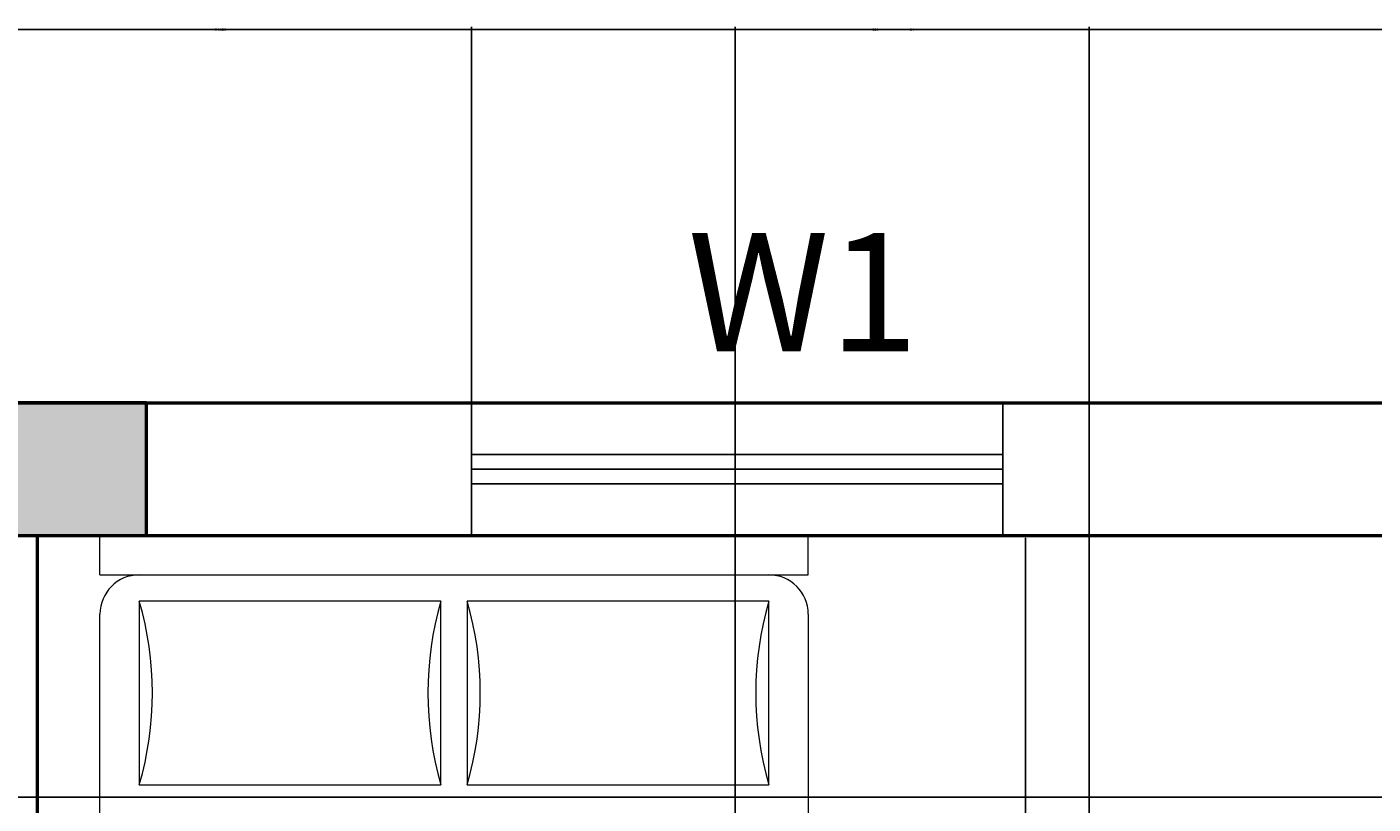
# Model space of a CAD drawing. Units: inches. Extents: x -1517 to -668, y -425 to 52.
# Tile 12 of 13: x -1186 to -1095, y -1 to 52. Entities that reach past the tile are written whole.
import ezdxf

# ---------------------------------------------------------------- set-up
doc = ezdxf.new("R2010")
doc.units = ezdxf.units.IN
doc.header["$MEASUREMENT"] = 0
for name, color, linetype, lineweight in [('A-ANNO-DIMS', 2, 'Continuous', 18), ('A-ANNO-TEXT', 7, 'Continuous', 18), ('A-COLS-PATT', 252, 'Continuous', 13), ('column', 7, 'Continuous', 50), ('furniture block', 8, 'Continuous', 18), ('walls', 240, 'Continuous', 50), ('windows', 140, 'Continuous', 25)]:
    doc.layers.add(name, color=color, linetype=linetype, lineweight=lineweight)
doc.styles.get("Standard").update_dxf_attribs({"font": 'arial.ttf'})
doc.dimstyles.get("Standard").update_dxf_attribs({"dimtxt": 0.18, "dimasz": 0.18, "dimexe": 0.18, "dimexo": 0.0625, "dimgap": 0.09, "dimtad": 0, "dimtih": 1, "dimtoh": 1, "dimdec": 4, "dimzin": 0, "dimdsep": 46, "dimlunit": 4, "dimtxsty": 'Standard', "dimcen": 0.09, "dimadec": 0, "dimazin": 0, "dimtfac": 1, "dimtdec": 4, "dimtofl": 0, "dimtmove": 0, "dimatfit": 3, "dimfxl": 1, "dimtolj": 1, "dimtzin": 0, "dimarcsym": 0})

# ---------------------------------------------------------------- blocks, each defined once
blk = doc.blocks.new('column')
for p, q in [((0, 9), (0, 0)), ((12, 9), (0, 9)), ((12, 0), (12, 9)), ((0, 0), (12, 0))]:
    blk.add_line(p, q)
blk = doc.blocks.new('window 3ft')
for p, q in [((9, 36), (0, 36)), ((3.5, 36), (3.5, 0)), ((4.5, 36), (4.5, 0)), ((5.5, 36), (5.5, 0)), ((9, 0), (0, 0))]:
    blk.add_line(p, q)
blk = doc.blocks.new('A$C62731D1C')
for p, q in [((0.0963, 2.2932, 0.6857), (1.4679, 2.2932, 0.6857)), ((0.0963, 2.217, 0.6857), (0.0963, 2.2932, 0.6857)), ((1.4679, 2.217, 0.6857), (1.4679, 2.2932, 0.6857)), ((0.0963, 2.217, 0.6857), (1.4679, 2.217, 0.6857)), ((0.7567, 2.1662, 0.6857), (0.1725, 2.1662, 0.6857)), ((0.1725, 2.1662, 0.6857), (0.1725, 1.8106, 0.6857)), ((0.7567, 1.8106, 0.6857), (0.7567, 2.1662, 0.6857)), ((0.8075, 2.1662, 0.6857), (0.8075, 1.8106, 0.6857)), ((1.3917, 2.1662, 0.6857), (0.8075, 2.1662, 0.6857)), ((1.3917, 1.8106, 0.6857), (1.3917, 2.1662, 0.6857)), ((0.0963, 0.3882, 0.6857), (0.0963, 2.1408, 0.6857)), ((1.4679, 2.1408, 0.6857), (1.4679, 0.3882, 0.6857)), ((0.1725, 1.8106, 0.6857), (0.7567, 1.8106, 0.6857)), ((0.8075, 1.8106, 0.6857), (1.3917, 1.8106, 0.6857))]:
    blk.add_line(p, q)
for centre, radius, start, end in [((0.1725, 2.1408, 0.6857), 0.0762, 90, 180), ((1.3917, 2.1408, 0.6857), 0.0762, 0, 90), ((-0.4371, 1.9884, 0.6857), 0.635, 343.7398, 16.2602), ((1.3663, 1.9884, 0.6857), 0.635, 163.7398, 196.2602), ((0.1979, 1.9884, 0.6857), 0.635, 343.7398, 16.2602), ((2.0013, 1.9884, 0.6857), 0.635, 163.7398, 196.2602)]:
    blk.add_arc(centre, radius, start, end)
blk = doc.blocks.new('A$C0E6D7E3D')
blk.add_blockref('A$C62731D1C', (0, 0))
blk = doc.blocks.new('*D36')
at = {"layer": 'A-ANNO-DIMS', "color": 0, "lineweight": -2, "transparency": 16777216}
for p, q in [((-1130.311, 17.63), (-1118.156, 17.63)), ((-1118.336, 17.45), (-1118.336, -22.314)), ((-1118.336, -62.443), (-1118.336, -22.68)), ((-1130.311, -62.623), (-1118.156, -62.623))]:
    blk.add_line(p, q, dxfattribs=at)
at = {"layer": 'A-ANNO-DIMS', "color": 0, "transparency": 16777216}
for points in [[(-1118.366, 17.45), (-1118.306, 17.45), (-1118.336, 17.63)], [(-1118.366, -62.443), (-1118.306, -62.443), (-1118.336, -62.623)]]:
    blk.add_solid(points, dxfattribs=at)
at = {"layer": 'Defpoints', "color": 0, "transparency": 16777216}
for p in [(-1130.374, 17.63), (-1118.336, 17.63), (-1130.374, -62.623)]:
    blk.add_point(p, dxfattribs=at)
at = {"layer": 'A-ANNO-DIMS', "color": 0, "transparency": 16777216, "insert": (-1118.336, -22.497), "char_height": 0.18, "attachment_point": 5}
blk.add_mtext("\\A1;CHILD'S BED 80", dxfattribs=at)
blk = doc.blocks.new('*D53')
at = {"layer": 'A-ANNO-DIMS', "color": 0, "lineweight": -2, "transparency": 16777216}
for p, q in [((-1242.504, -153.307), (-1242.504, 52.11)), ((-1014.504, -150.307), (-1014.504, 52.11)), ((-1242.324, 51.93), (-1128.794, 51.93)), ((-1014.684, 51.93), (-1128.213, 51.93))]:
    blk.add_line(p, q, dxfattribs=at)
at = {"layer": 'A-ANNO-DIMS', "color": 0, "transparency": 16777216}
for points in [[(-1242.324, 51.96), (-1242.324, 51.9), (-1242.504, 51.93)], [(-1014.684, 51.96), (-1014.684, 51.9), (-1014.504, 51.93)]]:
    blk.add_solid(points, dxfattribs=at)
at = {"layer": 'Defpoints', "color": 0, "transparency": 16777216}
for p in [(-1014.504, 51.93), (-1014.504, -150.37), (-1242.504, -153.37)]:
    blk.add_point(p, dxfattribs=at)
at = {"layer": 'A-ANNO-DIMS', "color": 0, "transparency": 16777216, "insert": (-1128.504, 51.93), "char_height": 0.18, "attachment_point": 5}
blk.add_mtext('\\A1;228', dxfattribs=at)
blk = doc.blocks.new('*D57')
at = {"layer": 'A-ANNO-DIMS', "color": 0, "lineweight": -2, "transparency": 16777216}
for p, q in [((-1114.018, -282.307), (-1114.018, 52.11)), ((-1066.018, -282.307), (-1066.018, 52.11)), ((-1113.838, 51.93), (-1090.241, 51.93)), ((-1066.198, 51.93), (-1089.796, 51.93))]:
    blk.add_line(p, q, dxfattribs=at)
at = {"layer": 'A-ANNO-DIMS', "color": 0, "transparency": 16777216}
for points in [[(-1113.838, 51.96), (-1113.838, 51.9), (-1114.018, 51.93)], [(-1066.198, 51.96), (-1066.198, 51.9), (-1066.018, 51.93)]]:
    blk.add_solid(points, dxfattribs=at)
at = {"layer": 'Defpoints', "color": 0, "transparency": 16777216}
for p in [(-1066.018, 51.93), (-1114.018, -282.37), (-1066.018, -282.37)]:
    blk.add_point(p, dxfattribs=at)
at = {"layer": 'A-ANNO-DIMS', "color": 0, "transparency": 16777216, "insert": (-1090.018, 51.93), "char_height": 0.18, "attachment_point": 5}
blk.add_mtext('\\A1;48', dxfattribs=at)
blk = doc.blocks.new('*D60')
at = {"layer": 'A-ANNO-DIMS', "color": 0, "lineweight": -2, "transparency": 16777216}
for p, q in [((-1189.904, 26.693), (-1189.904, 52.11)), ((-1155.878, 26.693), (-1155.878, 52.11)), ((-1189.724, 51.93), (-1173.355, 51.93)), ((-1156.058, 51.93), (-1172.427, 51.93))]:
    blk.add_line(p, q, dxfattribs=at)
at = {"layer": 'A-ANNO-DIMS', "color": 0, "transparency": 16777216}
for points in [[(-1189.724, 51.96), (-1189.724, 51.9), (-1189.904, 51.93)], [(-1156.058, 51.96), (-1156.058, 51.9), (-1155.878, 51.93)]]:
    blk.add_solid(points, dxfattribs=at)
at = {"layer": 'Defpoints', "color": 0, "transparency": 16777216}
for p in [(-1155.878, 51.93), (-1189.904, 26.63), (-1155.878, 26.63)]:
    blk.add_point(p, dxfattribs=at)
at = {"layer": 'A-ANNO-DIMS', "color": 0, "transparency": 16777216, "insert": (-1172.891, 51.93), "char_height": 0.18, "attachment_point": 5}
blk.add_mtext('\\A1;34.025', dxfattribs=at)
blk = doc.blocks.new('*D65')
at = {"layer": 'A-ANNO-DIMS', "color": 0, "lineweight": -2, "transparency": 16777216}
for p, q in [((-1138.018, -282.307), (-1138.018, 52.11)), ((-1114.018, -282.307), (-1114.018, 52.11)), ((-1137.838, 51.93), (-1126.238, 51.93)), ((-1114.198, 51.93), (-1125.798, 51.93))]:
    blk.add_line(p, q, dxfattribs=at)
at = {"layer": 'A-ANNO-DIMS', "color": 0, "transparency": 16777216}
for points in [[(-1137.838, 51.96), (-1137.838, 51.9), (-1138.018, 51.93)], [(-1114.198, 51.96), (-1114.198, 51.9), (-1114.018, 51.93)]]:
    blk.add_solid(points, dxfattribs=at)
at = {"layer": 'Defpoints', "color": 0, "transparency": 16777216}
for p in [(-1114.018, 51.93), (-1138.018, -282.37), (-1114.018, -282.37)]:
    blk.add_point(p, dxfattribs=at)
at = {"layer": 'A-ANNO-DIMS', "color": 0, "transparency": 16777216, "insert": (-1126.018, 51.93), "char_height": 0.18, "attachment_point": 5}
blk.add_mtext('\\A1;24', dxfattribs=at)
blk = doc.blocks.new('*D77')
at = {"layer": 'A-ANNO-DIMS', "color": 0, "lineweight": -2, "transparency": 16777216}
for p, q in [((-1482.441, 17.63), (-980.024, 17.63)), ((-980.204, 17.45), (-980.204, 8.938)), ((-980.204, 0.066), (-980.204, 8.578)), ((-1482.441, -0.114), (-980.024, -0.114))]:
    blk.add_line(p, q, dxfattribs=at)
at = {"layer": 'A-ANNO-DIMS', "color": 0, "transparency": 16777216}
for points in [[(-980.234, 17.45), (-980.174, 17.45), (-980.204, 17.63)], [(-980.234, 0.066), (-980.174, 0.066), (-980.204, -0.114)]]:
    blk.add_solid(points, dxfattribs=at)
at = {"layer": 'Defpoints', "color": 0, "transparency": 16777216}
for p in [(-1482.504, 17.63), (-1482.504, -0.114), (-980.204, -0.114)]:
    blk.add_point(p, dxfattribs=at)
at = {"layer": 'A-ANNO-DIMS', "color": 0, "transparency": 16777216, "insert": (-980.204, 8.758), "char_height": 0.18, "attachment_point": 5}
blk.add_mtext('\\A1;17.744', dxfattribs=at)

msp = doc.modelspace()

# ---------------------------------------------------------------- hatches: boundary and pattern name
at = {"layer": 'A-COLS-PATT'}
h = msp.add_hatch(dxfattribs=at)
h.set_pattern_fill('AR-CONC', color=256, scale=0.69)
h.set_pattern_definition([(50, (0, 0), (4.949095, -0.43299), [0.5175, -5.6925]), (355, (0, 0), (-0.957384, 5.190126), [0.414, -4.554]), (100.45144, (0.4124, -0.036), (3.991711, 4.757136), [0.439807, -4.83788]), (46.1842, (0, 1.38), (7.363965, -1.142083), [0.77625, -8.53875]), (96.63564, (0.614, 1.285), (6.449167, 6.72142), [0.65971, -7.256825]), (351.18416, (0, 1.38), (6.449167, 6.72142), [0.621, -6.831]), (21, (0.69, 1.035), (4.118659, -2.77807), [0.5175, -5.6925]), (326, (0.69, 1.035), (1.678876, 5.003535), [0.414, -4.554]), (71.45144, (1.033, 0.8035), (5.797534, 2.225465), [0.439807, -4.83788]), (37.5, (0, 0), (0.083903, 2.2969676), [0, -4.4988, 0, -4.623, 0, -4.57125]), (7.5, (0, 0), (1.81518, 2.721441), [0, -2.6358, 0, -4.3953, 0, -1.74225]), (327.5, (-1.5387, 0), (3.6833748, -0.1556286), [0, -1.725, 0, -5.382, 0, -7.1415]), (317.5, (-2.2287, 0), (4.0239846, 0.6907244), [0, -2.2425, 0, -3.5742, 0, -5.0715])])
h.paths.add_polyline_path([(-1491.5037, 26.63), (-1491.5037, 17.63), (-1479.5037, 17.63), (-1479.5037, 26.63)])
h.paths.add_polyline_path([(-1278.5037, 17.63), (-1278.5037, 26.63), (-1290.5037, 26.63), (-1290.5037, 17.63)])
h.paths.add_polyline_path([(-1177.9037, 26.63), (-1189.9037, 26.63), (-1189.9037, 17.63), (-1177.9037, 17.63)])
h.paths.add_polyline_path([(-1017.5037, 26.63), (-1017.5037, 17.63), (-1005.5037, 17.63), (-1005.5037, 26.63)])
h.paths.add_polyline_path([(-1005.5037, -270.37), (-1014.5037, -270.37), (-1014.5037, -282.37), (-1005.5037, -282.37)])
h.paths.add_polyline_path([(-1247.1037, -282.37), (-1235.1037, -282.37), (-1235.1037, -273.37), (-1247.1037, -273.37)])
h.paths.add_polyline_path([(-1367.1037, -273.37), (-1367.1037, -282.37), (-1355.1037, -282.37), (-1355.1037, -273.37)])
h.paths.add_polyline_path([(-1491.5037, -282.37), (-1479.5037, -282.37), (-1479.5037, -273.37), (-1491.5037, -273.37)])
h.paths.add_polyline_path([(-1482.5037, -145.97), (-1491.5037, -145.97), (-1491.5037, -157.97), (-1482.5037, -157.97)])
h.paths.add_polyline_path([(-1491.5037, -94.97), (-1491.5037, -106.97), (-1482.5037, -106.97), (-1482.5037, -94.97)])

# ---------------------------------------------------------------- linework, layer by layer
at = {"layer": 'walls'}
for p, q in [((-1491.5037, 26.63), (-1005.5037, 26.63)), ((-1185.3037, -102.37), (-1185.3037, 17.63)), ((-1185.3037, 17.63), (-1089.3037, 17.63))]:
    msp.add_line(p, q, dxfattribs=at)

# ---------------------------------------------------------------- block references
at = {"layer": 'column'}
msp.add_blockref('column', (-1189.9037, 17.63), dxfattribs=at)
at = {"layer": 'furniture block', "xscale": 34.99562554665724, "yscale": 34.99562554665724, "zscale": 34.99562554665724}
msp.add_blockref('A$C0E6D7E3D', (-1184.4382, -62.6234), dxfattribs=at)
at = {"layer": 'windows', "rotation": 270}
msp.add_blockref('window 3ft', (-1155.8782, 26.63), dxfattribs=at)

# ---------------------------------------------------------------- texts
at = {"layer": 'A-ANNO-TEXT', "insert": (-1141.2255, 38.1284), "char_height": 8, "attachment_point": 1}
msp.add_mtext_dynamic_manual_height_columns('{\\fArial|b1|i0|c0|p34;W1}', width=23.131632, gutter_width=1, heights=[0], dxfattribs=at)

# ---------------------------------------------------------------- dimensions: what is measured, and where the dimension line sits
at = {"layer": 'A-ANNO-DIMS'}
for base, p1, p2, override, picture, middle in [((-1014.5037, 51.93), (-1242.5037, -153.37), (-1014.5037, -150.37), {"dimdec": 0, "dimlfac": 1, "dimrnd": 0, "dimzin": 0, "dimdsep": 46, "dimlunit": 2}, '*D53', (-1128.5037, 51.93)), ((-1155.87819, 51.93001), (-1189.90368, 26.63001), (-1155.87819, 26.63001), {"dimdec": 3, "dimlfac": 1, "dimrnd": 0, "dimzin": 0, "dimdsep": 46, "dimlunit": 2}, '*D60', (-1172.89093, 51.93001)), ((-1114.0183, 51.93), (-1138.0183, -282.37), (-1114.0183, -282.37), {"dimdec": 0, "dimlfac": 1, "dimrnd": 0, "dimzin": 0, "dimdsep": 46, "dimlunit": 2}, '*D65', (-1126.0183, 51.93)), ((-1066.0183, 51.93), (-1114.0183, -282.37), (-1066.0183, -282.37), {"dimdec": 0, "dimlfac": 1, "dimrnd": 0, "dimzin": 0, "dimdsep": 46, "dimlunit": 2}, '*D57', (-1090.0183, 51.93))]:
    dim = msp.add_linear_dim(base=base, p1=p1, p2=p2, dimstyle='Standard', override=override, dxfattribs=at)
    dim.commit()
    dim.dimension.update_dxf_attribs({"geometry": picture, "text_midpoint": middle})
dim = msp.add_linear_dim(base=(-980.2037, -0.1142), p1=(-1482.5037, 17.63), p2=(-1482.5037, -0.1142), angle=90, dimstyle='Standard', override={"dimdec": 3, "dimlfac": 1, "dimrnd": 0, "dimzin": 0, "dimdsep": 46, "dimlunit": 2}, dxfattribs=at)
dim.commit()
dim.dimension.update_dxf_attribs({"geometry": '*D77', "text_midpoint": (-980.2037, 8.7579)})
dim = msp.add_linear_dim(base=(-1118.336, 17.63), p1=(-1130.374, -62.6234), p2=(-1130.374, 17.63), angle=90, text="CHILD'S BED <>", dimstyle='Standard', override={"dimdec": 0, "dimlfac": 1, "dimrnd": 0, "dimzin": 0, "dimdsep": 46, "dimlunit": 2}, dxfattribs=at)
dim.commit()
dim.dimension.update_dxf_attribs({"geometry": '*D36', "text_midpoint": (-1118.336, -22.4967)})

doc.saveas('drawing.dxf')
